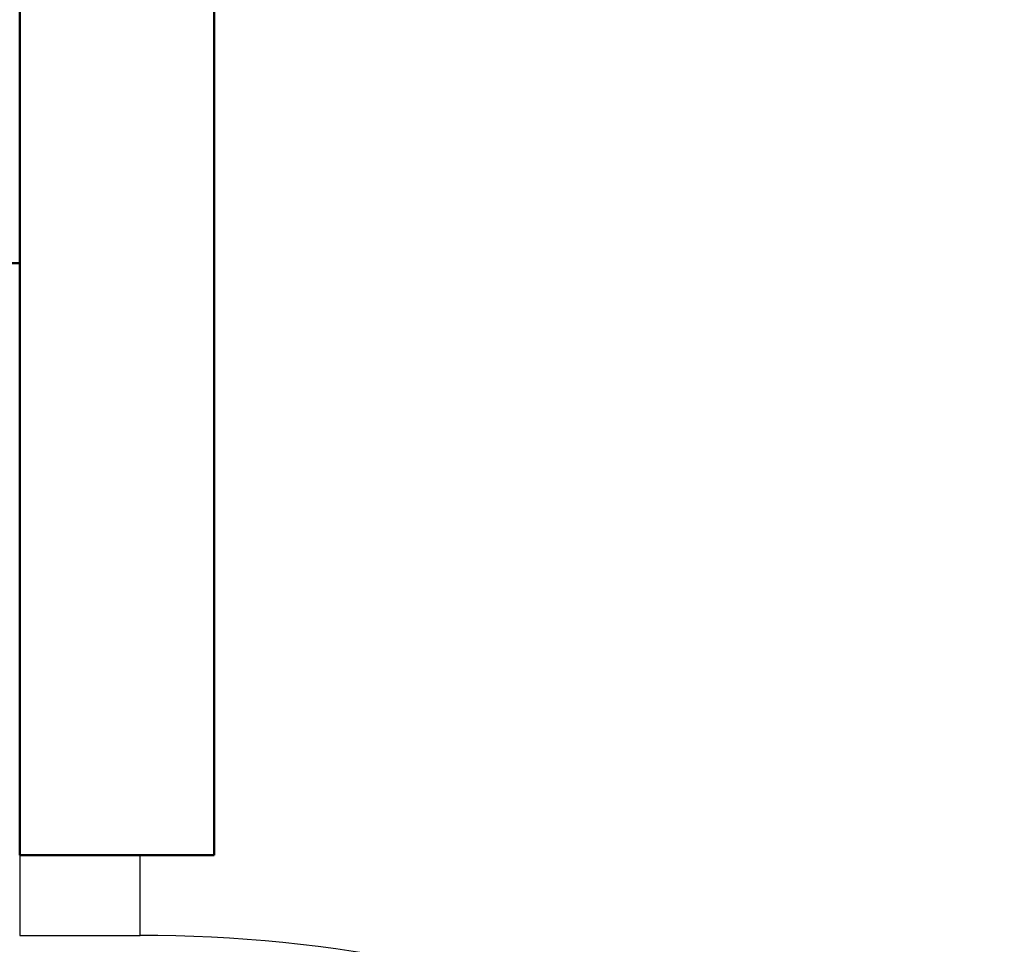
# Model space of a CAD drawing. Units: inches. Extents: x 64 to 1167, y 117 to 939.
# Tile 14 of 56: x 179 to 199, y 819 to 838. Entities that reach past the tile are written whole.
import ezdxf

# ---------------------------------------------------------------- set-up
doc = ezdxf.new("R2010")
doc.units = ezdxf.units.IN
doc.header["$MEASUREMENT"] = 0
doc.layers.add('A-DOOR', color=4, linetype='Continuous', lineweight=25)
doc.layers.add('A-WALL', color=7, linetype='Continuous', lineweight=50)

# ---------------------------------------------------------------- blocks, each defined once
blk = doc.blocks.new('A$C68901CC0')
for p, q in [((0, 2.953), (0, 0)), ((1.969, 2.953), (0, 2.953)), ((1.969, 0), (1.969, 2.953)), ((0, 0), (1.969, 0))]:
    blk.add_line(p, q)
blk.add_arc((37.402, 2.953), 35.433, 135, 180)

msp = doc.modelspace()

# ---------------------------------------------------------------- linework, layer by layer
at = {"layer": 'A-WALL'}
for p, q in [((179.107, 857.2), (179.107, 821.03)), ((183.107, 857.2), (183.107, 821.03)), ((179.107, 833.2), (131.107, 833.2)), ((183.107, 821.03), (179.107, 821.03))]:
    msp.add_line(p, q, dxfattribs=at)

# ---------------------------------------------------------------- block references
at = {"layer": 'A-DOOR', "xscale": 0.837864491618382, "yscale": 0.837864491618382, "zscale": 0.837864491618382, "rotation": 270}
msp.add_blockref('A$C68901CC0', (179.107, 821.03), dxfattribs=at)

doc.saveas('drawing.dxf')
